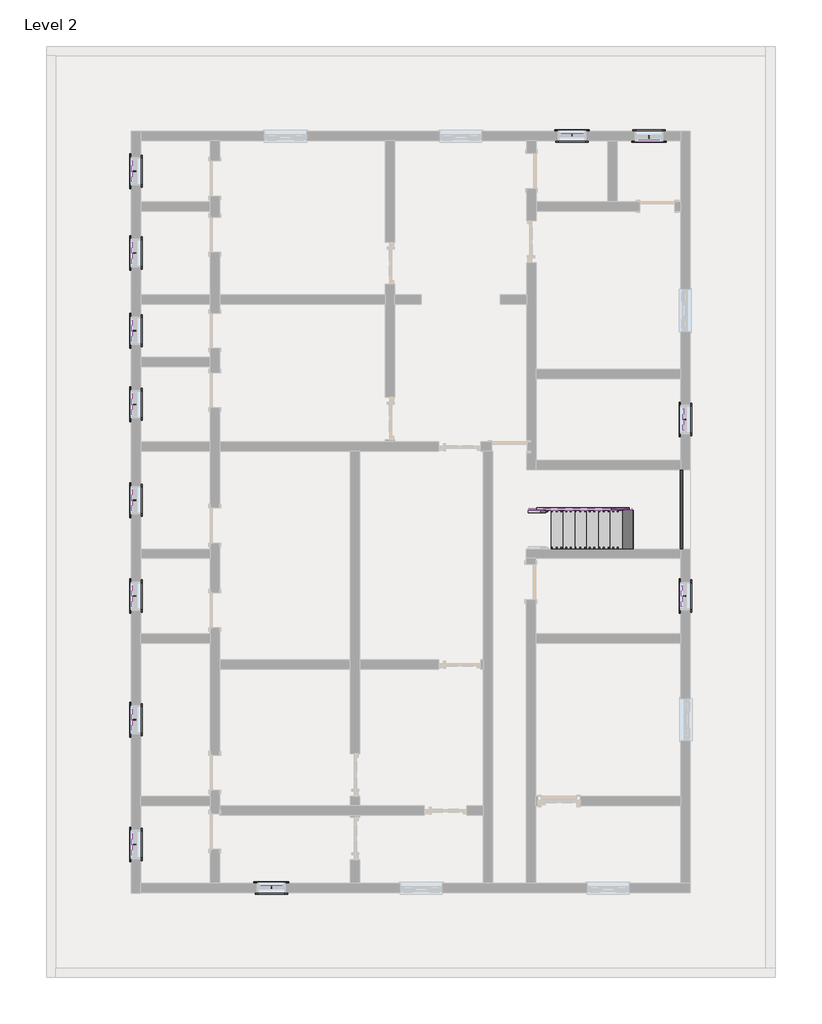
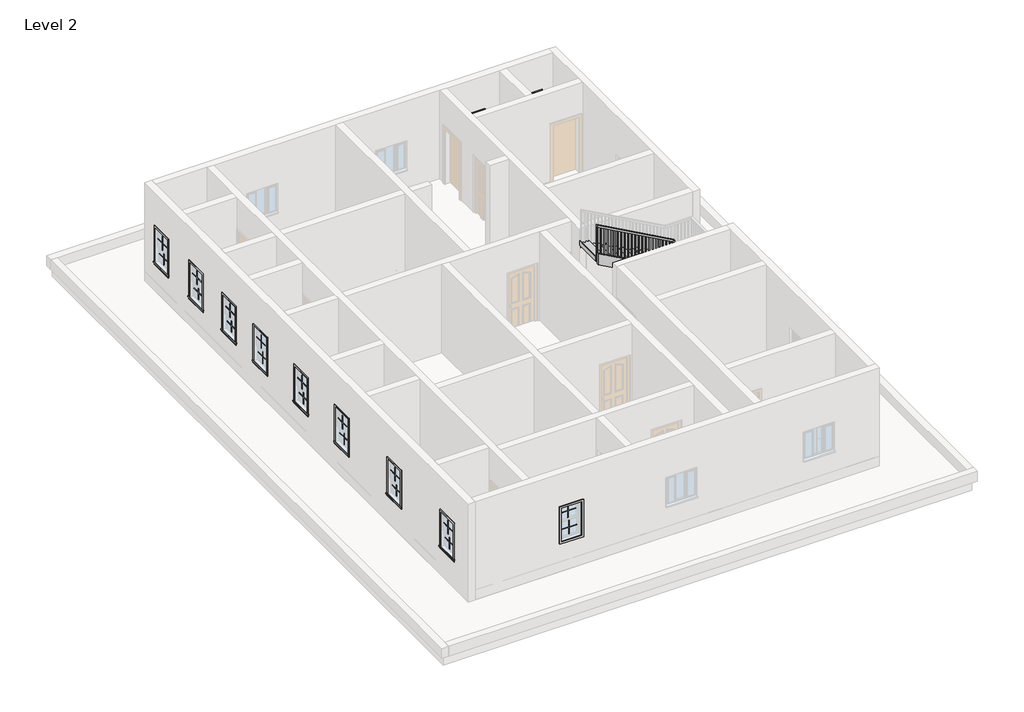
# One storey, part 3 of 3: 52 proxies, 5 members, 1 railing, 1 stair flight.
"""IFC4 building model written with IfcOpenShell, lengths in millimetres."""

from ifc_helpers import new_model, si_unit, frame, origin, place, context, project, spatial, polyline, outline, extrude, faceted_brep, transform, mapped, element, save
from components import muntin_pattern_2x2_muntin_pattern_2x2_eba6c5fb, trim_window_exterior_flat_with_sill_278e6a94, trim_window_interior_flat_picture_frame_e9fd5f45, stair_flight_45fd387a

model = new_model("IFC4")

# Units and contexts
model_context = context("Model", 3, world=origin())
ifc_project = project(units=[si_unit("LENGTHUNIT", "METRE", prefix="MILLI")], contexts=[model_context])

# Site, building, storey
site = spatial("IfcSite", under=ifc_project)
building = spatial("IfcBuilding", under=site)
storey = spatial("IfcBuildingStorey", under=building, Name="Level 2", Elevation=3048.0)

# Proxies
placement = place(None, origin())
muntin_pattern_2x2_muntin_pattern_2x2_shape = muntin_pattern_2x2_muntin_pattern_2x2_eba6c5fb(model_context)
element("IfcBuildingElementProxy", 1, Name="Muntin Pattern_2x2 : Muntin Pattern_2x2", ObjectType="Muntin Pattern_2x2 : Muntin Pattern_2x2", at=placement, inside=storey, context=model_context, shape_type="MappedRepresentation", body=[
    mapped(muntin_pattern_2x2_muntin_pattern_2x2_shape, transform((-10440.7626145, 6547.3404944, 4518.025), x_axis=(0.0, 1.0, 0.0), y_axis=(-1.0, 0.0, 0.0), z_axis=(0.0, 0.0, 1.0))),
])
element("IfcBuildingElementProxy", 2, Name="Muntin Pattern_2x2 : Muntin Pattern_2x2", ObjectType="Muntin Pattern_2x2 : Muntin Pattern_2x2", at=placement, inside=storey, context=model_context, shape_type="MappedRepresentation", body=[
    mapped(muntin_pattern_2x2_muntin_pattern_2x2_shape, transform((-10396.3126145, 6547.3404944, 4038.6), x_axis=(0.0, 1.0, 0.0), y_axis=(-1.0, 0.0, 0.0), z_axis=(0.0, 0.0, 1.0))),
])
element("IfcBuildingElementProxy", 3, Name="Muntin Pattern_2x2 : Muntin Pattern_2x2", ObjectType="Muntin Pattern_2x2 : Muntin Pattern_2x2", at=placement, inside=storey, context=model_context, shape_type="MappedRepresentation", body=[
    mapped(muntin_pattern_2x2_muntin_pattern_2x2_shape, transform((-10440.7626145, 4782.0404944, 4518.025), x_axis=(0.0, 1.0, 0.0), y_axis=(-1.0, 0.0, 0.0), z_axis=(0.0, 0.0, 1.0))),
])
element("IfcBuildingElementProxy", 4, Name="Muntin Pattern_2x2 : Muntin Pattern_2x2", ObjectType="Muntin Pattern_2x2 : Muntin Pattern_2x2", at=placement, inside=storey, context=model_context, shape_type="MappedRepresentation", body=[
    mapped(muntin_pattern_2x2_muntin_pattern_2x2_shape, transform((-10396.3126145, 4782.0404944, 4038.6), x_axis=(0.0, 1.0, 0.0), y_axis=(-1.0, 0.0, 0.0), z_axis=(0.0, 0.0, 1.0))),
])
element("IfcBuildingElementProxy", 5, Name="Muntin Pattern_2x2 : Muntin Pattern_2x2", ObjectType="Muntin Pattern_2x2 : Muntin Pattern_2x2", at=placement, inside=storey, context=model_context, shape_type="MappedRepresentation", body=[
    mapped(muntin_pattern_2x2_muntin_pattern_2x2_shape, transform((-10440.7626145, 3105.6404944, 4518.025), x_axis=(0.0, 1.0, 0.0), y_axis=(-1.0, 0.0, 0.0), z_axis=(0.0, 0.0, 1.0))),
])
element("IfcBuildingElementProxy", 6, Name="Muntin Pattern_2x2 : Muntin Pattern_2x2", ObjectType="Muntin Pattern_2x2 : Muntin Pattern_2x2", at=placement, inside=storey, context=model_context, shape_type="MappedRepresentation", body=[
    mapped(muntin_pattern_2x2_muntin_pattern_2x2_shape, transform((-10396.3126145, 3105.6404944, 4038.6), x_axis=(0.0, 1.0, 0.0), y_axis=(-1.0, 0.0, 0.0), z_axis=(0.0, 0.0, 1.0))),
])
element("IfcBuildingElementProxy", 7, Name="Muntin Pattern_2x2 : Muntin Pattern_2x2", ObjectType="Muntin Pattern_2x2 : Muntin Pattern_2x2", at=placement, inside=storey, context=model_context, shape_type="MappedRepresentation", body=[
    mapped(muntin_pattern_2x2_muntin_pattern_2x2_shape, transform((-10440.7626145, 1518.1404944, 4518.025), x_axis=(0.0, 1.0, 0.0), y_axis=(-1.0, 0.0, 0.0), z_axis=(0.0, 0.0, 1.0))),
])
element("IfcBuildingElementProxy", 8, Name="Muntin Pattern_2x2 : Muntin Pattern_2x2", ObjectType="Muntin Pattern_2x2 : Muntin Pattern_2x2", at=placement, inside=storey, context=model_context, shape_type="MappedRepresentation", body=[
    mapped(muntin_pattern_2x2_muntin_pattern_2x2_shape, transform((-10396.3126145, 1518.1404944, 4038.6), x_axis=(0.0, 1.0, 0.0), y_axis=(-1.0, 0.0, 0.0), z_axis=(0.0, 0.0, 1.0))),
])
element("IfcBuildingElementProxy", 9, Name="Muntin Pattern_2x2 : Muntin Pattern_2x2", ObjectType="Muntin Pattern_2x2 : Muntin Pattern_2x2", at=placement, inside=storey, context=model_context, shape_type="MappedRepresentation", body=[
    mapped(muntin_pattern_2x2_muntin_pattern_2x2_shape, transform((-10440.7626145, -551.9595056, 4518.025), x_axis=(0.0, 1.0, 0.0), y_axis=(-1.0, 0.0, 0.0), z_axis=(0.0, 0.0, 1.0))),
])
element("IfcBuildingElementProxy", 10, Name="Muntin Pattern_2x2 : Muntin Pattern_2x2", ObjectType="Muntin Pattern_2x2 : Muntin Pattern_2x2", at=placement, inside=storey, context=model_context, shape_type="MappedRepresentation", body=[
    mapped(muntin_pattern_2x2_muntin_pattern_2x2_shape, transform((-10396.3126145, -551.9595056, 4038.6), x_axis=(0.0, 1.0, 0.0), y_axis=(-1.0, 0.0, 0.0), z_axis=(0.0, 0.0, 1.0))),
])
element("IfcBuildingElementProxy", 11, Name="Muntin Pattern_2x2 : Muntin Pattern_2x2", ObjectType="Muntin Pattern_2x2 : Muntin Pattern_2x2", at=placement, inside=storey, context=model_context, shape_type="MappedRepresentation", body=[
    mapped(muntin_pattern_2x2_muntin_pattern_2x2_shape, transform((-10440.7626145, -2622.0595056, 4518.025), x_axis=(0.0, 1.0, 0.0), y_axis=(-1.0, 0.0, 0.0), z_axis=(0.0, 0.0, 1.0))),
])
element("IfcBuildingElementProxy", 12, Name="Muntin Pattern_2x2 : Muntin Pattern_2x2", ObjectType="Muntin Pattern_2x2 : Muntin Pattern_2x2", at=placement, inside=storey, context=model_context, shape_type="MappedRepresentation", body=[
    mapped(muntin_pattern_2x2_muntin_pattern_2x2_shape, transform((-10396.3126145, -2622.0595056, 4038.6), x_axis=(0.0, 1.0, 0.0), y_axis=(-1.0, 0.0, 0.0), z_axis=(0.0, 0.0, 1.0))),
])
element("IfcBuildingElementProxy", 13, Name="Muntin Pattern_2x2 : Muntin Pattern_2x2", ObjectType="Muntin Pattern_2x2 : Muntin Pattern_2x2", at=placement, inside=storey, context=model_context, shape_type="MappedRepresentation", body=[
    mapped(muntin_pattern_2x2_muntin_pattern_2x2_shape, transform((-10440.7626145, -5289.0595056, 4518.025), x_axis=(0.0, 1.0, 0.0), y_axis=(-1.0, 0.0, 0.0), z_axis=(0.0, 0.0, 1.0))),
])
element("IfcBuildingElementProxy", 14, Name="Muntin Pattern_2x2 : Muntin Pattern_2x2", ObjectType="Muntin Pattern_2x2 : Muntin Pattern_2x2", at=placement, inside=storey, context=model_context, shape_type="MappedRepresentation", body=[
    mapped(muntin_pattern_2x2_muntin_pattern_2x2_shape, transform((-10396.3126145, -5289.0595056, 4038.6), x_axis=(0.0, 1.0, 0.0), y_axis=(-1.0, 0.0, 0.0), z_axis=(0.0, 0.0, 1.0))),
])
element("IfcBuildingElementProxy", 15, Name="Muntin Pattern_2x2 : Muntin Pattern_2x2", ObjectType="Muntin Pattern_2x2 : Muntin Pattern_2x2", at=placement, inside=storey, context=model_context, shape_type="MappedRepresentation", body=[
    mapped(muntin_pattern_2x2_muntin_pattern_2x2_shape, transform((-10440.7626145, -7981.4595056, 4518.025), x_axis=(0.0, 1.0, 0.0), y_axis=(-1.0, 0.0, 0.0), z_axis=(0.0, 0.0, 1.0))),
])
element("IfcBuildingElementProxy", 16, Name="Muntin Pattern_2x2 : Muntin Pattern_2x2", ObjectType="Muntin Pattern_2x2 : Muntin Pattern_2x2", at=placement, inside=storey, context=model_context, shape_type="MappedRepresentation", body=[
    mapped(muntin_pattern_2x2_muntin_pattern_2x2_shape, transform((-10396.3126145, -7981.4595056, 4038.6), x_axis=(0.0, 1.0, 0.0), y_axis=(-1.0, 0.0, 0.0), z_axis=(0.0, 0.0, 1.0))),
])
element("IfcBuildingElementProxy", 17, Name="Muntin Pattern_2x2 : Muntin Pattern_2x2", ObjectType="Muntin Pattern_2x2 : Muntin Pattern_2x2", at=placement, inside=storey, context=model_context, shape_type="MappedRepresentation", body=[
    mapped(muntin_pattern_2x2_muntin_pattern_2x2_shape, transform((-7453.0876145, -8854.5845056, 4518.025), x_axis=(1.0, 0.0, 0.0), y_axis=(0.0, 1.0, 0.0), z_axis=(0.0, 0.0, 1.0))),
])
element("IfcBuildingElementProxy", 18, Name="Muntin Pattern_2x2 : Muntin Pattern_2x2", ObjectType="Muntin Pattern_2x2 : Muntin Pattern_2x2", at=placement, inside=storey, context=model_context, shape_type="MappedRepresentation", body=[
    mapped(muntin_pattern_2x2_muntin_pattern_2x2_shape, transform((-7453.0876145, -8899.0345056, 4038.6), x_axis=(1.0, 0.0, 0.0), y_axis=(0.0, 1.0, 0.0), z_axis=(0.0, 0.0, 1.0))),
])
element("IfcBuildingElementProxy", 19, Name="Muntin Pattern_2x2 : Muntin Pattern_2x2", ObjectType="Muntin Pattern_2x2 : Muntin Pattern_2x2", at=placement, inside=storey, context=model_context, shape_type="MappedRepresentation", body=[
    mapped(muntin_pattern_2x2_muntin_pattern_2x2_shape, transform((1421.0373855, -2622.0595056, 4518.025), x_axis=(0.0, 1.0, 0.0), y_axis=(-1.0, 0.0, 0.0), z_axis=(0.0, 0.0, 1.0))),
])
element("IfcBuildingElementProxy", 20, Name="Muntin Pattern_2x2 : Muntin Pattern_2x2", ObjectType="Muntin Pattern_2x2 : Muntin Pattern_2x2", at=placement, inside=storey, context=model_context, shape_type="MappedRepresentation", body=[
    mapped(muntin_pattern_2x2_muntin_pattern_2x2_shape, transform((1465.4873855, -2622.0595056, 4038.6), x_axis=(0.0, 1.0, 0.0), y_axis=(-1.0, 0.0, 0.0), z_axis=(0.0, 0.0, 1.0))),
])
element("IfcBuildingElementProxy", 21, Name="Muntin Pattern_2x2 : Muntin Pattern_2x2", ObjectType="Muntin Pattern_2x2 : Muntin Pattern_2x2", at=placement, inside=storey, context=model_context, shape_type="MappedRepresentation", body=[
    mapped(muntin_pattern_2x2_muntin_pattern_2x2_shape, transform((1421.0373855, 1190.4645364, 4518.025), x_axis=(0.0, 1.0, 0.0), y_axis=(-1.0, 0.0, 0.0), z_axis=(0.0, 0.0, 1.0))),
])
element("IfcBuildingElementProxy", 22, Name="Muntin Pattern_2x2 : Muntin Pattern_2x2", ObjectType="Muntin Pattern_2x2 : Muntin Pattern_2x2", at=placement, inside=storey, context=model_context, shape_type="MappedRepresentation", body=[
    mapped(muntin_pattern_2x2_muntin_pattern_2x2_shape, transform((1465.4873855, 1190.4645364, 4038.6), x_axis=(0.0, 1.0, 0.0), y_axis=(-1.0, 0.0, 0.0), z_axis=(0.0, 0.0, 1.0))),
])
element("IfcBuildingElementProxy", 23, Name="Muntin Pattern_2x2 : Muntin Pattern_2x2", ObjectType="Muntin Pattern_2x2 : Muntin Pattern_2x2", at=placement, inside=storey, context=model_context, shape_type="MappedRepresentation", body=[
    mapped(muntin_pattern_2x2_muntin_pattern_2x2_shape, transform((700.3123855, 7242.6654944, 4518.025), x_axis=(-1.0, 0.0, 0.0), y_axis=(0.0, -1.0, 0.0), z_axis=(0.0, 0.0, 1.0))),
])
element("IfcBuildingElementProxy", 24, Name="Muntin Pattern_2x2 : Muntin Pattern_2x2", ObjectType="Muntin Pattern_2x2 : Muntin Pattern_2x2", at=placement, inside=storey, context=model_context, shape_type="MappedRepresentation", body=[
    mapped(muntin_pattern_2x2_muntin_pattern_2x2_shape, transform((700.3123855, 7287.1154944, 4038.6), x_axis=(-1.0, 0.0, 0.0), y_axis=(0.0, -1.0, 0.0), z_axis=(0.0, 0.0, 1.0))),
])
element("IfcBuildingElementProxy", 25, Name="Muntin Pattern_2x2 : Muntin Pattern_2x2", ObjectType="Muntin Pattern_2x2 : Muntin Pattern_2x2", at=placement, inside=storey, context=model_context, shape_type="MappedRepresentation", body=[
    mapped(muntin_pattern_2x2_muntin_pattern_2x2_shape, transform((-963.3876145, 7376.0154944, 4518.025), x_axis=(1.0, 0.0, 0.0), y_axis=(0.0, 1.0, 0.0), z_axis=(0.0, 0.0, 1.0))),
])
element("IfcBuildingElementProxy", 26, Name="Muntin Pattern_2x2 : Muntin Pattern_2x2", ObjectType="Muntin Pattern_2x2 : Muntin Pattern_2x2", at=placement, inside=storey, context=model_context, shape_type="MappedRepresentation", body=[
    mapped(muntin_pattern_2x2_muntin_pattern_2x2_shape, transform((-963.3876145, 7331.5654944, 4038.6), x_axis=(1.0, 0.0, 0.0), y_axis=(0.0, 1.0, 0.0), z_axis=(0.0, 0.0, 1.0))),
])
trim_window_exterior_flat_with_sill_shape = trim_window_exterior_flat_with_sill_278e6a94(model_context)
element("IfcBuildingElementProxy", 27, Name="Trim-Window-Exterior-Flat : with Sill", ObjectType="Trim-Window-Exterior-Flat : with Sill", at=placement, inside=storey, context=model_context, shape_type="MappedRepresentation", body=[
    mapped(trim_window_exterior_flat_with_sill_shape, transform((-10475.6876145, 6547.3404944, 5029.2), x_axis=(0.0, -1.0, 0.0), y_axis=(0.0, 0.0, 1.0), z_axis=(-1.0, 0.0, 0.0))),
])
element("IfcBuildingElementProxy", 28, Name="Trim-Window-Exterior-Flat : with Sill", ObjectType="Trim-Window-Exterior-Flat : with Sill", at=placement, inside=storey, context=model_context, shape_type="MappedRepresentation", body=[
    mapped(trim_window_exterior_flat_with_sill_shape, transform((-10475.6876145, 4782.0404944, 5029.2), x_axis=(0.0, -1.0, 0.0), y_axis=(0.0, 0.0, 1.0), z_axis=(-1.0, 0.0, 0.0))),
])
element("IfcBuildingElementProxy", 29, Name="Trim-Window-Exterior-Flat : with Sill", ObjectType="Trim-Window-Exterior-Flat : with Sill", at=placement, inside=storey, context=model_context, shape_type="MappedRepresentation", body=[
    mapped(trim_window_exterior_flat_with_sill_shape, transform((-10475.6876145, 3105.6404944, 5029.2), x_axis=(0.0, -1.0, 0.0), y_axis=(0.0, 0.0, 1.0), z_axis=(-1.0, 0.0, 0.0))),
])
element("IfcBuildingElementProxy", 30, Name="Trim-Window-Exterior-Flat : with Sill", ObjectType="Trim-Window-Exterior-Flat : with Sill", at=placement, inside=storey, context=model_context, shape_type="MappedRepresentation", body=[
    mapped(trim_window_exterior_flat_with_sill_shape, transform((-10475.6876145, 1518.1404944, 5029.2), x_axis=(0.0, -1.0, 0.0), y_axis=(0.0, 0.0, 1.0), z_axis=(-1.0, 0.0, 0.0))),
])
element("IfcBuildingElementProxy", 31, Name="Trim-Window-Exterior-Flat : with Sill", ObjectType="Trim-Window-Exterior-Flat : with Sill", at=placement, inside=storey, context=model_context, shape_type="MappedRepresentation", body=[
    mapped(trim_window_exterior_flat_with_sill_shape, transform((-10475.6876145, -551.9595056, 5029.2), x_axis=(0.0, -1.0, 0.0), y_axis=(0.0, 0.0, 1.0), z_axis=(-1.0, 0.0, 0.0))),
])
element("IfcBuildingElementProxy", 32, Name="Trim-Window-Exterior-Flat : with Sill", ObjectType="Trim-Window-Exterior-Flat : with Sill", at=placement, inside=storey, context=model_context, shape_type="MappedRepresentation", body=[
    mapped(trim_window_exterior_flat_with_sill_shape, transform((-10475.6876145, -2622.0595056, 5029.2), x_axis=(0.0, -1.0, 0.0), y_axis=(0.0, 0.0, 1.0), z_axis=(-1.0, 0.0, 0.0))),
])
element("IfcBuildingElementProxy", 33, Name="Trim-Window-Exterior-Flat : with Sill", ObjectType="Trim-Window-Exterior-Flat : with Sill", at=placement, inside=storey, context=model_context, shape_type="MappedRepresentation", body=[
    mapped(trim_window_exterior_flat_with_sill_shape, transform((-10475.6876145, -5289.0595056, 5029.2), x_axis=(0.0, -1.0, 0.0), y_axis=(0.0, 0.0, 1.0), z_axis=(-1.0, 0.0, 0.0))),
])
element("IfcBuildingElementProxy", 34, Name="Trim-Window-Exterior-Flat : with Sill", ObjectType="Trim-Window-Exterior-Flat : with Sill", at=placement, inside=storey, context=model_context, shape_type="MappedRepresentation", body=[
    mapped(trim_window_exterior_flat_with_sill_shape, transform((-10475.6876145, -7981.4595056, 5029.2), x_axis=(0.0, -1.0, 0.0), y_axis=(0.0, 0.0, 1.0), z_axis=(-1.0, 0.0, 0.0))),
])
element("IfcBuildingElementProxy", 35, Name="Trim-Window-Exterior-Flat : with Sill", ObjectType="Trim-Window-Exterior-Flat : with Sill", at=placement, inside=storey, context=model_context, shape_type="MappedRepresentation", body=[
    mapped(trim_window_exterior_flat_with_sill_shape, transform((-7453.0876145, -8819.6595056, 5029.2), x_axis=(-1.0, 0.0, 0.0), y_axis=(0.0, 0.0, 1.0), z_axis=(0.0, 1.0, 0.0))),
])
element("IfcBuildingElementProxy", 36, Name="Trim-Window-Exterior-Flat : with Sill", ObjectType="Trim-Window-Exterior-Flat : with Sill", at=placement, inside=storey, context=model_context, shape_type="MappedRepresentation", body=[
    mapped(trim_window_exterior_flat_with_sill_shape, transform((1386.1123855, -2622.0595056, 5029.2), x_axis=(0.0, -1.0, 0.0), y_axis=(0.0, 0.0, 1.0), z_axis=(-1.0, 0.0, 0.0))),
])
element("IfcBuildingElementProxy", 37, Name="Trim-Window-Exterior-Flat : with Sill", ObjectType="Trim-Window-Exterior-Flat : with Sill", at=placement, inside=storey, context=model_context, shape_type="MappedRepresentation", body=[
    mapped(trim_window_exterior_flat_with_sill_shape, transform((1386.1123855, 1190.4645364, 5029.2), x_axis=(0.0, -1.0, 0.0), y_axis=(0.0, 0.0, 1.0), z_axis=(-1.0, 0.0, 0.0))),
])
element("IfcBuildingElementProxy", 38, Name="Trim-Window-Exterior-Flat : with Sill", ObjectType="Trim-Window-Exterior-Flat : with Sill", at=placement, inside=storey, context=model_context, shape_type="MappedRepresentation", body=[
    mapped(trim_window_exterior_flat_with_sill_shape, transform((700.3123855, 7207.7404944, 5029.2), x_axis=(1.0, 0.0, 0.0), y_axis=(0.0, 0.0, 1.0), z_axis=(0.0, -1.0, 0.0))),
])
element("IfcBuildingElementProxy", 39, Name="Trim-Window-Exterior-Flat : with Sill", ObjectType="Trim-Window-Exterior-Flat : with Sill", at=placement, inside=storey, context=model_context, shape_type="MappedRepresentation", body=[
    mapped(trim_window_exterior_flat_with_sill_shape, transform((-963.3876145, 7410.9404944, 5029.2), x_axis=(-1.0, 0.0, 0.0), y_axis=(0.0, 0.0, 1.0), z_axis=(0.0, 1.0, 0.0))),
])
trim_window_interior_flat_picture_frame_shape = trim_window_interior_flat_picture_frame_e9fd5f45(model_context)
element("IfcBuildingElementProxy", 40, Name="Trim-Window-Interior-Flat : Picture Frame", ObjectType="Trim-Window-Interior-Flat : Picture Frame", at=placement, inside=storey, context=model_context, shape_type="MappedRepresentation", body=[
    mapped(trim_window_interior_flat_picture_frame_shape, transform((-10272.4876145, 6547.3404944, 5029.2), x_axis=(0.0, 1.0, 0.0), y_axis=(0.0, 0.0, 1.0), z_axis=(1.0, 0.0, 0.0))),
])
element("IfcBuildingElementProxy", 41, Name="Trim-Window-Interior-Flat : Picture Frame", ObjectType="Trim-Window-Interior-Flat : Picture Frame", at=placement, inside=storey, context=model_context, shape_type="MappedRepresentation", body=[
    mapped(trim_window_interior_flat_picture_frame_shape, transform((-10272.4876145, 4782.0404944, 5029.2), x_axis=(0.0, 1.0, 0.0), y_axis=(0.0, 0.0, 1.0), z_axis=(1.0, 0.0, 0.0))),
])
element("IfcBuildingElementProxy", 42, Name="Trim-Window-Interior-Flat : Picture Frame", ObjectType="Trim-Window-Interior-Flat : Picture Frame", at=placement, inside=storey, context=model_context, shape_type="MappedRepresentation", body=[
    mapped(trim_window_interior_flat_picture_frame_shape, transform((-10272.4876145, 3105.6404944, 5029.2), x_axis=(0.0, 1.0, 0.0), y_axis=(0.0, 0.0, 1.0), z_axis=(1.0, 0.0, 0.0))),
])
element("IfcBuildingElementProxy", 43, Name="Trim-Window-Interior-Flat : Picture Frame", ObjectType="Trim-Window-Interior-Flat : Picture Frame", at=placement, inside=storey, context=model_context, shape_type="MappedRepresentation", body=[
    mapped(trim_window_interior_flat_picture_frame_shape, transform((-10272.4876145, 1518.1404944, 5029.2), x_axis=(0.0, 1.0, 0.0), y_axis=(0.0, 0.0, 1.0), z_axis=(1.0, 0.0, 0.0))),
])
element("IfcBuildingElementProxy", 44, Name="Trim-Window-Interior-Flat : Picture Frame", ObjectType="Trim-Window-Interior-Flat : Picture Frame", at=placement, inside=storey, context=model_context, shape_type="MappedRepresentation", body=[
    mapped(trim_window_interior_flat_picture_frame_shape, transform((-10272.4876145, -551.9595056, 5029.2), x_axis=(0.0, 1.0, 0.0), y_axis=(0.0, 0.0, 1.0), z_axis=(1.0, 0.0, 0.0))),
])
element("IfcBuildingElementProxy", 45, Name="Trim-Window-Interior-Flat : Picture Frame", ObjectType="Trim-Window-Interior-Flat : Picture Frame", at=placement, inside=storey, context=model_context, shape_type="MappedRepresentation", body=[
    mapped(trim_window_interior_flat_picture_frame_shape, transform((-10272.4876145, -2622.0595056, 5029.2), x_axis=(0.0, 1.0, 0.0), y_axis=(0.0, 0.0, 1.0), z_axis=(1.0, 0.0, 0.0))),
])
element("IfcBuildingElementProxy", 46, Name="Trim-Window-Interior-Flat : Picture Frame", ObjectType="Trim-Window-Interior-Flat : Picture Frame", at=placement, inside=storey, context=model_context, shape_type="MappedRepresentation", body=[
    mapped(trim_window_interior_flat_picture_frame_shape, transform((-10272.4876145, -5289.0595056, 5029.2), x_axis=(0.0, 1.0, 0.0), y_axis=(0.0, 0.0, 1.0), z_axis=(1.0, 0.0, 0.0))),
])
element("IfcBuildingElementProxy", 47, Name="Trim-Window-Interior-Flat : Picture Frame", ObjectType="Trim-Window-Interior-Flat : Picture Frame", at=placement, inside=storey, context=model_context, shape_type="MappedRepresentation", body=[
    mapped(trim_window_interior_flat_picture_frame_shape, transform((-10272.4876145, -7981.4595056, 5029.2), x_axis=(0.0, 1.0, 0.0), y_axis=(0.0, 0.0, 1.0), z_axis=(1.0, 0.0, 0.0))),
])
element("IfcBuildingElementProxy", 48, Name="Trim-Window-Interior-Flat : Picture Frame", ObjectType="Trim-Window-Interior-Flat : Picture Frame", at=placement, inside=storey, context=model_context, shape_type="MappedRepresentation", body=[
    mapped(trim_window_interior_flat_picture_frame_shape, transform((-7453.0876145, -9022.8595056, 5029.2), x_axis=(1.0, 0.0, 0.0), y_axis=(0.0, 0.0, 1.0), z_axis=(0.0, -1.0, 0.0))),
])
element("IfcBuildingElementProxy", 49, Name="Trim-Window-Interior-Flat : Picture Frame", ObjectType="Trim-Window-Interior-Flat : Picture Frame", at=placement, inside=storey, context=model_context, shape_type="MappedRepresentation", body=[
    mapped(trim_window_interior_flat_picture_frame_shape, transform((1589.3123855, -2622.0595056, 5029.2), x_axis=(0.0, 1.0, 0.0), y_axis=(0.0, 0.0, 1.0), z_axis=(1.0, 0.0, 0.0))),
])
element("IfcBuildingElementProxy", 50, Name="Trim-Window-Interior-Flat : Picture Frame", ObjectType="Trim-Window-Interior-Flat : Picture Frame", at=placement, inside=storey, context=model_context, shape_type="MappedRepresentation", body=[
    mapped(trim_window_interior_flat_picture_frame_shape, transform((1589.3123855, 1190.4645364, 5029.2), x_axis=(0.0, 1.0, 0.0), y_axis=(0.0, 0.0, 1.0), z_axis=(1.0, 0.0, 0.0))),
])
element("IfcBuildingElementProxy", 51, Name="Trim-Window-Interior-Flat : Picture Frame", ObjectType="Trim-Window-Interior-Flat : Picture Frame", at=placement, inside=storey, context=model_context, shape_type="MappedRepresentation", body=[
    mapped(trim_window_interior_flat_picture_frame_shape, transform((700.3123855, 7410.9404944, 5029.2), x_axis=(-1.0, 0.0, 0.0), y_axis=(0.0, 0.0, 1.0), z_axis=(0.0, 1.0, 0.0))),
])
element("IfcBuildingElementProxy", 52, Name="Trim-Window-Interior-Flat : Picture Frame", ObjectType="Trim-Window-Interior-Flat : Picture Frame", at=placement, inside=storey, context=model_context, shape_type="MappedRepresentation", body=[
    mapped(trim_window_interior_flat_picture_frame_shape, transform((-963.3876145, 7207.7404944, 5029.2), x_axis=(1.0, 0.0, 0.0), y_axis=(0.0, 0.0, 1.0), z_axis=(0.0, -1.0, 0.0))),
])

# Members
element("IfcMember", 53, ObjectType="Stringer - 2\" Width", at=placement, inside=storey, context=model_context, shape_type="SweptSolid", body=[
    extrude(outline(polyline([(3258.6757607, -1903.1876145), (3048.0, -1903.1876145), (3048.0, -1654.2050647), (4113.4963497, 274.6830625), (4461.7073019, 274.6830625), (3258.6757607, -1903.1876145)])), frame((0.0, -767.8595056, 0.0), z_axis=(0.0, 1.0, 0.0), x_axis=(0.0, 0.0, 1.0)), (0.0, 0.0, 1.0), 50.8),
])
element("IfcMember", 54, ObjectType="Stringer - 2\" Width", at=placement, inside=storey, context=model_context, shape_type="SweptSolid", body=[
    extrude(outline(polyline([(4278.7177047, 325.4830625), (4626.928657, 325.4830625), (5858.0215532, -1903.1876145), (5509.8106009, -1903.1876145), (4278.7177047, 325.4830625)])), frame((0.0, -780.5595056, 0.0), z_axis=(0.0, 1.0, 0.0), x_axis=(0.0, 0.0, 1.0)), (0.0, 0.0, 1.0), 50.8),
])
element("IfcMember", 55, ObjectType="Stringer - 2\" Width", at=placement, inside=storey, context=model_context, shape_type="SweptSolid", body=[
    extrude(outline(polyline([(3258.6757607, -1903.1876145), (3048.0, -1903.1876145), (3048.0, -1654.2050647), (4495.8, 966.7745674), (4495.8, 336.4017165), (3258.6757607, -1903.1876145)])), frame((0.0, -1656.8595056, 0.0), z_axis=(0.0, 1.0, 0.0), x_axis=(0.0, 0.0, 1.0)), (0.0, 0.0, 1.0), 50.8),
])
element("IfcMember", 56, ObjectType="Stringer - 2\" Width", at=placement, inside=storey, context=model_context, shape_type="SweptSolid", body=[
    extrude(outline(polyline([(1424.2123855, -1656.8595056), (1373.4123855, -1656.8595056), (1373.4123855, 108.4404944), (1424.2123855, 108.4404944), (1424.2123855, -1656.8595056)])), frame((0.0, 0.0, 4191.0), z_axis=(0.0, 0.0, 1.0), x_axis=(1.0, 0.0, 0.0)), (0.0, 0.0, 1.0), 304.8),
])
element("IfcMember", 57, ObjectType="Stringer - 2\" Width", at=placement, inside=storey, context=model_context, shape_type="SweptSolid", body=[
    extrude(outline(polyline([(4191.0, 1114.6529278), (5858.0215532, -1903.1876145), (5509.8106009, -1903.1876145), (4191.0, 484.2800769), (4191.0, 1114.6529278)])), frame((0.0, 108.4404944, 0.0), z_axis=(0.0, 1.0, 0.0), x_axis=(0.0, 0.0, 1.0)), (0.0, 0.0, 1.0), 50.8),
])

# Railing
element("IfcRailing", 58, ObjectType="Handrail - Rectangular", at=placement, inside=storey, context=model_context, shape_type="SolidModel", body=[
    faceted_brep([(-1903.1876145, -767.8595056, 4099.56), (-1903.1876145, -767.8595056, 4041.4879132), (-1903.1876145, -818.6595056, 4041.4879132), (-1903.1876145, -818.6595056, 4099.56), (325.4830625, -767.8595056, 5334.0), (325.4830625, -818.6595056, 5334.0), (325.4830625, -818.6595056, 5275.9279132), (325.4830625, -767.8595056, 5275.9279132)], [[[0, 1, 2, 3]], [[4, 5, 6, 7]], [[1, 0, 4, 7]], [[2, 1, 7, 6]], [[3, 2, 6, 5]], [[0, 3, 5, 4]]]),
    faceted_brep([(325.4830625, -818.6595056, 5334.0), (325.4830625, -818.6595056, 5283.2), (376.2830625, -818.6595056, 5283.2), (376.2830625, -818.6595056, 5334.0), (325.4830625, -729.7595056, 5334.0), (376.2830625, -729.7595056, 5334.0), (376.2830625, -678.9595056, 5283.2), (325.4830625, -678.9595056, 5283.2)], [[[0, 1, 2, 3]], [[4, 5, 6, 7]], [[1, 0, 4, 7]], [[2, 1, 7, 6]], [[3, 2, 6, 5]], [[0, 3, 5, 4]]]),
    faceted_brep([(325.4830625, -729.7595056, 5334.0), (325.4830625, -678.9595056, 5283.2), (376.2830625, -678.9595056, 5283.2), (376.2830625, -729.7595056, 5334.0), (325.4830625, -729.7595056, 5413.0879132), (376.2830625, -729.7595056, 5443.0223516), (376.2830625, -678.9595056, 5443.0223516), (325.4830625, -678.9595056, 5413.0879132)], [[[0, 1, 2, 3]], [[4, 5, 6, 7]], [[1, 0, 4, 7]], [[2, 1, 7, 6]], [[3, 2, 6, 5]], [[0, 3, 5, 4]]]),
    faceted_brep([(376.2830625, -729.7595056, 5443.0223516), (325.4830625, -729.7595056, 5413.0879132), (325.4830625, -678.9595056, 5413.0879132), (376.2830625, -678.9595056, 5443.0223516), (-1903.1876145, -729.7595056, 6705.6), (-1903.1876145, -678.9595056, 6705.6), (-1903.1876145, -678.9595056, 6647.5279132), (-1903.1876145, -729.7595056, 6647.5279132)], [[[0, 1, 2, 3]], [[4, 5, 6, 7]], [[1, 0, 4, 7]], [[2, 1, 7, 6]], [[3, 2, 6, 5]], [[0, 3, 5, 4]]]),
    extrude(outline(polyline([(6642.3072849, -1893.8419375), (5654.04, -1893.8419375), (5654.04, -1874.7919375), (6631.7556667, -1874.7919375), (6642.3072849, -1893.8419375)])), frame((0.0, -713.8845056, 0.0), z_axis=(0.0, 1.0, 0.0), x_axis=(0.0, 0.0, 1.0)), (0.0, 0.0, 1.0), 19.05),
    extrude(outline(polyline([(6586.031988, -1792.2419375), (5654.04, -1792.2419375), (5654.04, -1773.1919375), (6575.4803699, -1773.1919375), (6586.031988, -1792.2419375)])), frame((0.0, -713.8845056, 0.0), z_axis=(0.0, 1.0, 0.0), x_axis=(0.0, 0.0, 1.0)), (0.0, 0.0, 1.0), 19.05),
    extrude(outline(polyline([(6529.7125465, -1690.6419375), (5654.04, -1690.6419375), (5654.04, -1671.5919375), (6519.1609284, -1671.5919375), (6529.7125465, -1690.6419375)])), frame((0.0, -713.8845056, 0.0), z_axis=(0.0, 1.0, 0.0), x_axis=(0.0, 0.0, 1.0)), (0.0, 0.0, 1.0), 19.05),
    extrude(outline(polyline([(6473.4813943, -1589.0419375), (5516.88, -1589.0419375), (5516.88, -1569.9919375), (6462.9297761, -1569.9919375), (6473.4813943, -1589.0419375)])), frame((0.0, -713.8845056, 0.0), z_axis=(0.0, 1.0, 0.0), x_axis=(0.0, 0.0, 1.0)), (0.0, 0.0, 1.0), 19.05),
    extrude(outline(polyline([(6417.2060974, -1487.4419375), (5516.88, -1487.4419375), (5516.88, -1468.3919375), (6406.6544792, -1468.3919375), (6417.2060974, -1487.4419375)])), frame((0.0, -713.8845056, 0.0), z_axis=(0.0, 1.0, 0.0), x_axis=(0.0, 0.0, 1.0)), (0.0, 0.0, 1.0), 19.05),
    extrude(outline(polyline([(6360.9308005, -1385.8419375), (5379.72, -1385.8419375), (5379.72, -1366.7919375), (6350.3791823, -1366.7919375), (6360.9308005, -1385.8419375)])), frame((0.0, -713.8845056, 0.0), z_axis=(0.0, 1.0, 0.0), x_axis=(0.0, 0.0, 1.0)), (0.0, 0.0, 1.0), 19.05),
    extrude(outline(polyline([(6304.6555036, -1284.2419375), (5379.72, -1284.2419375), (5379.72, -1265.1919375), (6294.1038855, -1265.1919375), (6304.6555036, -1284.2419375)])), frame((0.0, -713.8845056, 0.0), z_axis=(0.0, 1.0, 0.0), x_axis=(0.0, 0.0, 1.0)), (0.0, 0.0, 1.0), 19.05),
    extrude(outline(polyline([(6248.3802067, -1182.6419375), (5379.72, -1182.6419375), (5379.72, -1163.5919375), (6237.8285886, -1163.5919375), (6248.3802067, -1182.6419375)])), frame((0.0, -713.8845056, 0.0), z_axis=(0.0, 1.0, 0.0), x_axis=(0.0, 0.0, 1.0)), (0.0, 0.0, 1.0), 19.05),
    extrude(outline(polyline([(6192.1049099, -1081.0419375), (5242.56, -1081.0419375), (5242.56, -1061.9919375), (6181.5532917, -1061.9919375), (6192.1049099, -1081.0419375)])), frame((0.0, -713.8845056, 0.0), z_axis=(0.0, 1.0, 0.0), x_axis=(0.0, 0.0, 1.0)), (0.0, 0.0, 1.0), 19.05),
    extrude(outline(polyline([(6135.829613, -979.4419375), (5242.56, -979.4419375), (5242.56, -960.3919375), (6125.2779948, -960.3919375), (6135.829613, -979.4419375)])), frame((0.0, -713.8845056, 0.0), z_axis=(0.0, 1.0, 0.0), x_axis=(0.0, 0.0, 1.0)), (0.0, 0.0, 1.0), 19.05),
    extrude(outline(polyline([(6079.5543161, -877.8419375), (5105.4, -877.8419375), (5105.4, -858.7919375), (6069.0026979, -858.7919375), (6079.5543161, -877.8419375)])), frame((0.0, -713.8845056, 0.0), z_axis=(0.0, 1.0, 0.0), x_axis=(0.0, 0.0, 1.0)), (0.0, 0.0, 1.0), 19.05),
    extrude(outline(polyline([(6023.2790192, -776.2419375), (5105.4, -776.2419375), (5105.4, -757.1919375), (6012.727401, -757.1919375), (6023.2790192, -776.2419375)])), frame((0.0, -713.8845056, 0.0), z_axis=(0.0, 1.0, 0.0), x_axis=(0.0, 0.0, 1.0)), (0.0, 0.0, 1.0), 19.05),
    extrude(outline(polyline([(5967.0478669, -674.6419375), (5105.4, -674.6419375), (5105.4, -655.5919375), (5956.4962488, -655.5919375), (5967.0478669, -674.6419375)])), frame((0.0, -713.8845056, 0.0), z_axis=(0.0, 1.0, 0.0), x_axis=(0.0, 0.0, 1.0)), (0.0, 0.0, 1.0), 19.05),
    extrude(outline(polyline([(5910.77257, -573.0419375), (4968.24, -573.0419375), (4968.24, -553.9919375), (5900.2209519, -553.9919375), (5910.77257, -573.0419375)])), frame((0.0, -713.8845056, 0.0), z_axis=(0.0, 1.0, 0.0), x_axis=(0.0, 0.0, 1.0)), (0.0, 0.0, 1.0), 19.05),
    extrude(outline(polyline([(5854.4972732, -471.4419375), (4968.24, -471.4419375), (4968.24, -452.3919375), (5843.945655, -452.3919375), (5854.4972732, -471.4419375)])), frame((0.0, -713.8845056, 0.0), z_axis=(0.0, 1.0, 0.0), x_axis=(0.0, 0.0, 1.0)), (0.0, 0.0, 1.0), 19.05),
    extrude(outline(polyline([(5798.2219763, -369.8419375), (4831.08, -369.8419375), (4831.08, -350.7919375), (5787.6703581, -350.7919375), (5798.2219763, -369.8419375)])), frame((0.0, -713.8845056, 0.0), z_axis=(0.0, 1.0, 0.0), x_axis=(0.0, 0.0, 1.0)), (0.0, 0.0, 1.0), 19.05),
    extrude(outline(polyline([(5741.9466794, -268.2419375), (4831.08, -268.2419375), (4831.08, -249.1919375), (5731.3950612, -249.1919375), (5741.9466794, -268.2419375)])), frame((0.0, -713.8845056, 0.0), z_axis=(0.0, 1.0, 0.0), x_axis=(0.0, 0.0, 1.0)), (0.0, 0.0, 1.0), 19.05),
    extrude(outline(polyline([(5685.6713825, -166.6419375), (4831.08, -166.6419375), (4831.08, -147.5919375), (5675.1197643, -147.5919375), (5685.6713825, -166.6419375)])), frame((0.0, -713.8845056, 0.0), z_axis=(0.0, 1.0, 0.0), x_axis=(0.0, 0.0, 1.0)), (0.0, 0.0, 1.0), 19.05),
    extrude(outline(polyline([(5629.3960856, -65.0419375), (4693.92, -65.0419375), (4693.92, -45.9919375), (5618.8444675, -45.9919375), (5629.3960856, -65.0419375)])), frame((0.0, -713.8845056, 0.0), z_axis=(0.0, 1.0, 0.0), x_axis=(0.0, 0.0, 1.0)), (0.0, 0.0, 1.0), 19.05),
    extrude(outline(polyline([(5573.1207888, 36.5580625), (4693.92, 36.5580625), (4693.92, 55.6080625), (5562.5691706, 55.6080625), (5573.1207888, 36.5580625)])), frame((0.0, -713.8845056, 0.0), z_axis=(0.0, 1.0, 0.0), x_axis=(0.0, 0.0, 1.0)), (0.0, 0.0, 1.0), 19.05),
    extrude(outline(polyline([(5516.8454919, 138.1580625), (4556.76, 138.1580625), (4556.76, 157.2080625), (5506.2938737, 157.2080625), (5516.8454919, 138.1580625)])), frame((0.0, -713.8845056, 0.0), z_axis=(0.0, 1.0, 0.0), x_axis=(0.0, 0.0, 1.0)), (0.0, 0.0, 1.0), 19.05),
    extrude(outline(polyline([(5460.570195, 239.7580625), (4556.76, 239.7580625), (4556.76, 258.8080625), (5450.0185768, 258.8080625), (5460.570195, 239.7580625)])), frame((0.0, -713.8845056, 0.0), z_axis=(0.0, 1.0, 0.0), x_axis=(0.0, 0.0, 1.0)), (0.0, 0.0, 1.0), 19.05),
    extrude(outline(polyline([(5274.2686355, 322.4873855), (4419.6, 322.4873855), (4419.6, 341.5373855), (5284.8202537, 341.5373855), (5274.2686355, 322.4873855)])), frame((0.0, -802.7845056, 0.0), z_axis=(0.0, 1.0, 0.0), x_axis=(0.0, 0.0, 1.0)), (0.0, 0.0, 1.0), 19.05),
    extrude(outline(polyline([(5217.9933387, 220.8873855), (4282.44, 220.8873855), (4282.44, 239.9373855), (5228.5449568, 239.9373855), (5217.9933387, 220.8873855)])), frame((0.0, -802.7845056, 0.0), z_axis=(0.0, 1.0, 0.0), x_axis=(0.0, 0.0, 1.0)), (0.0, 0.0, 1.0), 19.05),
    extrude(outline(polyline([(5161.7180418, 119.2873855), (4282.44, 119.2873855), (4282.44, 138.3373855), (5172.2696599, 138.3373855), (5161.7180418, 119.2873855)])), frame((0.0, -802.7845056, 0.0), z_axis=(0.0, 1.0, 0.0), x_axis=(0.0, 0.0, 1.0)), (0.0, 0.0, 1.0), 19.05),
    extrude(outline(polyline([(5105.4427449, 17.6873855), (4145.28, 17.6873855), (4145.28, 36.7373855), (5115.9943631, 36.7373855), (5105.4427449, 17.6873855)])), frame((0.0, -802.7845056, 0.0), z_axis=(0.0, 1.0, 0.0), x_axis=(0.0, 0.0, 1.0)), (0.0, 0.0, 1.0), 19.05),
    extrude(outline(polyline([(5049.167448, -83.9126145), (4145.28, -83.9126145), (4145.28, -64.8626145), (5059.7190662, -64.8626145), (5049.167448, -83.9126145)])), frame((0.0, -802.7845056, 0.0), z_axis=(0.0, 1.0, 0.0), x_axis=(0.0, 0.0, 1.0)), (0.0, 0.0, 1.0), 19.05),
    extrude(outline(polyline([(4992.8921511, -185.5126145), (4008.12, -185.5126145), (4008.12, -166.4626145), (5003.4437693, -166.4626145), (4992.8921511, -185.5126145)])), frame((0.0, -802.7845056, 0.0), z_axis=(0.0, 1.0, 0.0), x_axis=(0.0, 0.0, 1.0)), (0.0, 0.0, 1.0), 19.05),
    extrude(outline(polyline([(4936.6168543, -287.1126145), (4008.12, -287.1126145), (4008.12, -268.0626145), (4947.1684724, -268.0626145), (4936.6168543, -287.1126145)])), frame((0.0, -802.7845056, 0.0), z_axis=(0.0, 1.0, 0.0), x_axis=(0.0, 0.0, 1.0)), (0.0, 0.0, 1.0), 19.05),
    extrude(outline(polyline([(4880.3415574, -388.7126145), (4008.12, -388.7126145), (4008.12, -369.6626145), (4890.8931755, -369.6626145), (4880.3415574, -388.7126145)])), frame((0.0, -802.7845056, 0.0), z_axis=(0.0, 1.0, 0.0), x_axis=(0.0, 0.0, 1.0)), (0.0, 0.0, 1.0), 19.05),
    extrude(outline(polyline([(4824.0662605, -490.3126145), (3870.96, -490.3126145), (3870.96, -471.2626145), (4834.6178787, -471.2626145), (4824.0662605, -490.3126145)])), frame((0.0, -802.7845056, 0.0), z_axis=(0.0, 1.0, 0.0), x_axis=(0.0, 0.0, 1.0)), (0.0, 0.0, 1.0), 19.05),
    extrude(outline(polyline([(4767.7909636, -591.9126145), (3870.96, -591.9126145), (3870.96, -572.8626145), (4778.3425818, -572.8626145), (4767.7909636, -591.9126145)])), frame((0.0, -802.7845056, 0.0), z_axis=(0.0, 1.0, 0.0), x_axis=(0.0, 0.0, 1.0)), (0.0, 0.0, 1.0), 19.05),
    extrude(outline(polyline([(4711.5156667, -693.5126145), (3733.8, -693.5126145), (3733.8, -674.4626145), (4722.0672849, -674.4626145), (4711.5156667, -693.5126145)])), frame((0.0, -802.7845056, 0.0), z_axis=(0.0, 1.0, 0.0), x_axis=(0.0, 0.0, 1.0)), (0.0, 0.0, 1.0), 19.05),
    extrude(outline(polyline([(4655.2403699, -795.1126145), (3733.8, -795.1126145), (3733.8, -776.0626145), (4665.791988, -776.0626145), (4655.2403699, -795.1126145)])), frame((0.0, -802.7845056, 0.0), z_axis=(0.0, 1.0, 0.0), x_axis=(0.0, 0.0, 1.0)), (0.0, 0.0, 1.0), 19.05),
    extrude(outline(polyline([(4598.9209284, -896.7126145), (3733.8, -896.7126145), (3733.8, -877.6626145), (4609.4725465, -877.6626145), (4598.9209284, -896.7126145)])), frame((0.0, -802.7845056, 0.0), z_axis=(0.0, 1.0, 0.0), x_axis=(0.0, 0.0, 1.0)), (0.0, 0.0, 1.0), 19.05),
    extrude(outline(polyline([(4542.6897761, -998.3126145), (3596.64, -998.3126145), (3596.64, -979.2626145), (4553.2413943, -979.2626145), (4542.6897761, -998.3126145)])), frame((0.0, -802.7845056, 0.0), z_axis=(0.0, 1.0, 0.0), x_axis=(0.0, 0.0, 1.0)), (0.0, 0.0, 1.0), 19.05),
    extrude(outline(polyline([(4486.4144792, -1099.9126145), (3596.64, -1099.9126145), (3596.64, -1080.8626145), (4496.9660974, -1080.8626145), (4486.4144792, -1099.9126145)])), frame((0.0, -802.7845056, 0.0), z_axis=(0.0, 1.0, 0.0), x_axis=(0.0, 0.0, 1.0)), (0.0, 0.0, 1.0), 19.05),
    extrude(outline(polyline([(4430.1391823, -1201.5126145), (3459.48, -1201.5126145), (3459.48, -1182.4626145), (4440.6908005, -1182.4626145), (4430.1391823, -1201.5126145)])), frame((0.0, -802.7845056, 0.0), z_axis=(0.0, 1.0, 0.0), x_axis=(0.0, 0.0, 1.0)), (0.0, 0.0, 1.0), 19.05),
    extrude(outline(polyline([(4373.8638855, -1303.1126145), (3459.48, -1303.1126145), (3459.48, -1284.0626145), (4384.4155036, -1284.0626145), (4373.8638855, -1303.1126145)])), frame((0.0, -802.7845056, 0.0), z_axis=(0.0, 1.0, 0.0), x_axis=(0.0, 0.0, 1.0)), (0.0, 0.0, 1.0), 19.05),
    extrude(outline(polyline([(4317.5885886, -1404.7126145), (3459.48, -1404.7126145), (3459.48, -1385.6626145), (4328.1402067, -1385.6626145), (4317.5885886, -1404.7126145)])), frame((0.0, -802.7845056, 0.0), z_axis=(0.0, 1.0, 0.0), x_axis=(0.0, 0.0, 1.0)), (0.0, 0.0, 1.0), 19.05),
    extrude(outline(polyline([(4261.3132917, -1506.3126145), (3322.32, -1506.3126145), (3322.32, -1487.2626145), (4271.8649099, -1487.2626145), (4261.3132917, -1506.3126145)])), frame((0.0, -802.7845056, 0.0), z_axis=(0.0, 1.0, 0.0), x_axis=(0.0, 0.0, 1.0)), (0.0, 0.0, 1.0), 19.05),
    extrude(outline(polyline([(4205.0379948, -1607.9126145), (3322.32, -1607.9126145), (3322.32, -1588.8626145), (4215.589613, -1588.8626145), (4205.0379948, -1607.9126145)])), frame((0.0, -802.7845056, 0.0), z_axis=(0.0, 1.0, 0.0), x_axis=(0.0, 0.0, 1.0)), (0.0, 0.0, 1.0), 19.05),
    extrude(outline(polyline([(4148.7626979, -1709.5126145), (3185.16, -1709.5126145), (3185.16, -1690.4626145), (4159.3143161, -1690.4626145), (4148.7626979, -1709.5126145)])), frame((0.0, -802.7845056, 0.0), z_axis=(0.0, 1.0, 0.0), x_axis=(0.0, 0.0, 1.0)), (0.0, 0.0, 1.0), 19.05),
    extrude(outline(polyline([(4092.487401, -1811.1126145), (3185.16, -1811.1126145), (3185.16, -1792.0626145), (4103.0390192, -1792.0626145), (4092.487401, -1811.1126145)])), frame((0.0, -802.7845056, 0.0), z_axis=(0.0, 1.0, 0.0), x_axis=(0.0, 0.0, 1.0)), (0.0, 0.0, 1.0), 19.05),
    extrude(outline(polyline([(341.3580625, -713.8845056), (341.3580625, -694.8345056), (360.4080625, -694.8345056), (360.4080625, -713.8845056), (341.3580625, -713.8845056)])), frame((0.0, 0.0, 4419.6), z_axis=(0.0, 0.0, 1.0), x_axis=(1.0, 0.0, 0.0)), (0.0, 0.0, 1.0), 863.6),
    extrude(outline(polyline([(5284.7209284, 341.3580625), (4419.6, 341.3580625), (4419.6, 360.4080625), (5295.2725465, 360.4080625), (5284.7209284, 341.3580625)])), frame((0.0, -802.7845056, 0.0), z_axis=(0.0, 1.0, 0.0), x_axis=(0.0, 0.0, 1.0)), (0.0, 0.0, 1.0), 19.05),
    extrude(outline(polyline([(6647.5279132, -1903.1876145), (5654.04, -1903.1876145), (5654.04, -1884.1376145), (6636.9762951, -1884.1376145), (6647.5279132, -1903.1876145)])), frame((0.0, -713.8845056, 0.0), z_axis=(0.0, 1.0, 0.0), x_axis=(0.0, 0.0, 1.0)), (0.0, 0.0, 1.0), 19.05),
    extrude(outline(polyline([(4041.4879132, -1903.1876145), (3185.16, -1903.1876145), (3185.16, -1884.1376145), (4052.0395314, -1884.1376145), (4041.4879132, -1903.1876145)])), frame((0.0, -802.7845056, 0.0), z_axis=(0.0, 1.0, 0.0), x_axis=(0.0, 0.0, 1.0)), (0.0, 0.0, 1.0), 19.05),
])

# Stair flight
stair_flight_shape = stair_flight_45fd387a(model_context)
element("IfcStairFlight", 59, ObjectType="2\" Tread 1\" Nosing 1/4\" Riser", at=placement, inside=storey, context=model_context, shape_type="MappedRepresentation", body=[
    mapped(stair_flight_shape, transform((0.0, 0.0, 0.0), x_axis=(1.0, 0.0, 0.0), y_axis=(0.0, 1.0, 0.0), z_axis=(0.0, 0.0, 1.0))),
])

save(model, "model.ifc")

# Revit data of these elements
# Type "Muntin Pattern_2x2 : Muntin Pattern_2x2"
#   Width [instance default] = 4' - 0"
#   Thickness = 0' - 0 1/2"
#   Height [instance default] = 4' - 0"
#   Distance = 0' - 0 3/4"
#   Interior Material [instance default] = none
#   Exterior Material [instance default] = none
#   Default Elevation = 0
# Type "Trim-Window-Exterior-Flat : with Sill"
#   Trim Width = 0' - 2 1/4"
#   Trim Thickness_Picture Frame = 0' - 1 1/4"
#   Trim Thickness_with Sill = 0' - 0 3/4"
#   Sill Thickness = 0' - 1 1/4"
#   Opening Width [instance default] = 2' - 0"
#   Opening Height [instance default] = 3' - 0"
#   Default Elevation = 4' - 0"
#   Sill = yes
#   Picture Frame = no
#   Trim Material [instance default] = none
# Type "Trim-Window-Interior-Flat : Picture Frame"
#   Trim Thickness_Picture Frame = 0' - 1 1/4"
#   Trim Width = 0' - 2 1/4"
#   Trim Thickness_with Sill = 0' - 0 3/4"
#   Sill Thickness = 0' - 1 1/4"
#   Opening Width [instance default] = 2' - 0"
#   Opening Height [instance default] = 3' - 0"
#   Default Elevation = 4' - 0"
#   Sill = no
#   Picture Frame = yes
#   Trim Material [instance default] = none
# Type "Handrail - Rectangular"
#   Assembly Code = "C2010400"
#   built-in parameter 1008612 = 0.0416667 (stored number, unit not read)
#   built-in parameter 1008611 = 0.0416667 (stored number, unit not read)
#   built-in parameter 1008609 = 0.333333 (stored number, unit not read)
#   built-in parameter 1008604 = 0.166667 (stored number, unit not read)
#   built-in parameter 1008603 = 0.166667 (stored number, unit not read)
#   Railing Height = 3' - 0"
#   built-in parameter 1008630 = 2
#   built-in parameter 1008610 = 2
#   built-in parameter 1008618 = Baluster - Square : 3/4"
# Elements 1, 2, 3, 4, 5, 6, 7, 8, 9, 10, 11, 12, 13, 14, 15, 16, 17, 18, 19, 20, 21, 22, 23, 24, 25, 26 (IfcBuildingElementProxy, "Muntin Pattern_2x2 : Muntin Pattern_2x2")
#   Width = 1' - 6"
#   Height = 1' - 5 1/8"
#   Interior Material = Wood - Stained
#   Exterior Material = Clad - White
#   Phase Created = New Construction
#   Materials on its faces: "Clad - White", "Wood - Stained"
# Elements 27, 28, 29, 30, 31, 32, 33, 34, 35, 36, 37, 38, 39 (IfcBuildingElementProxy, "Trim-Window-Exterior-Flat : with Sill")
#   Opening Width = 2' - 0"
#   Opening Height = 3' - 6"
#   Trim Material = Clad - White
#   Phase Created = New Construction
#   Materials on its faces: "Clad - White"
# Elements 40, 41, 42, 43, 44, 45, 46, 47, 48, 49, 50, 51, 52 (IfcBuildingElementProxy, "Trim-Window-Interior-Flat : Picture Frame")
#   Opening Width = 2' - 0"
#   Opening Height = 3' - 6"
#   Trim Material = Wood - Stained
#   Phase Created = New Construction
#   Materials on its faces: "Wood - Stained"
# Elements 53, 54, 55, 56, 57 (IfcMember, "Stringer - 2\" Width")
#   Phase Created = New Construction
# Element 58 (IfcRailing, "Handrail - Rectangular")
#   Phase Created = New Construction
# Element 59 (IfcStairFlight, "2\" Tread 1\" Nosing 1/4\" Riser")
#   Phase Created = New Construction
# Materials
#   "Clad - White": class "Wood", colour RGB 242 242 238, transparency 0, Cost = 0
#   "Wood - Stained": class "Wood", colour RGB 224 178 126, transparency 0, Cost = 0
